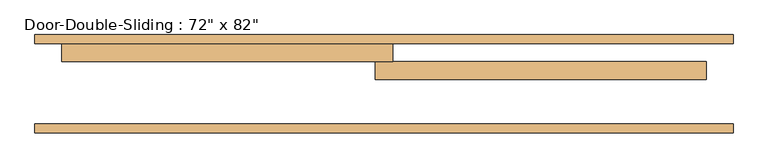
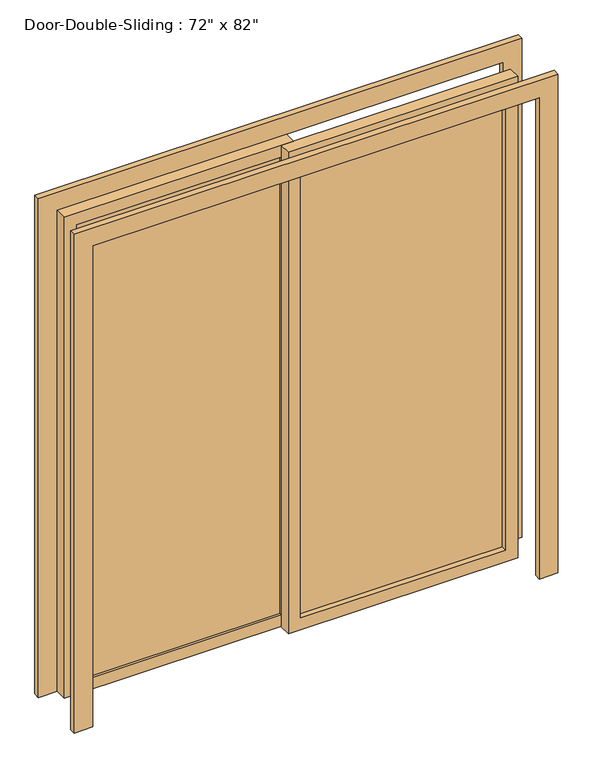
"""IFC4 building model written with IfcOpenShell, lengths in millimetres: door geometry."""

from ifc_helpers import new_model, si_unit, frame, origin, place, context, project, spatial, polyline, outline, extrude, source, transform, mapped, element, save


def door_b7c0cbe2(model_context):
    return source(origin(), model_context, "Body", "SweptSolid", [
        extrude(outline(polyline([(0.0, 990.6), (2159.0, 990.6), (2159.0, -990.6), (0.0, -990.6), (0.0, -914.4), (2082.8, -914.4), (2082.8, 914.4), (0.0, 914.4), (0.0, 990.6)])), frame((0.0, 241.3, 0.0), z_axis=(0.0, 1.0, 0.0), x_axis=(0.0, 0.0, 1.0)), (0.0, 0.0, 1.0), 25.4),
        extrude(outline(polyline([(0.0, -990.6), (0.0, -914.4), (2082.8, -914.4), (2082.8, 914.4), (0.0, 914.4), (0.0, 990.6), (2159.0, 990.6), (2159.0, -990.6), (0.0, -990.6)])), frame((0.0, -12.7, 0.0), z_axis=(0.0, 1.0, 0.0), x_axis=(0.0, 0.0, 1.0)), (0.0, 0.0, 1.0), 25.4),
        extrude(outline(polyline([(2082.8, 25.4), (2082.8, -914.4), (0.0, -914.4), (0.0, 25.4), (2082.8, 25.4)]), holes=[polyline([(2032.0, -25.4), (50.8, -25.4), (50.8, -863.6), (2032.0, -863.6), (2032.0, -25.4)])]), frame((0.0, 190.5, 0.0), z_axis=(0.0, 1.0, 0.0), x_axis=(0.0, 0.0, 1.0)), (0.0, 0.0, 1.0), 50.8),
        extrude(outline(polyline([(2082.8, -25.4), (0.0, -25.4), (0.0, 914.4), (2082.8, 914.4), (2082.8, -25.4)]), holes=[polyline([(2032.0, 25.4), (2032.0, 863.6), (50.8, 863.6), (50.8, 25.4), (2032.0, 25.4)])]), frame((0.0, 139.7, 0.0), z_axis=(0.0, 1.0, 0.0), x_axis=(0.0, 0.0, 1.0)), (0.0, 0.0, 1.0), 50.8),
        extrude(outline(polyline([(-25.4, 200.025), (-863.6, 200.025), (-863.6, 206.375), (-25.4, 206.375), (-25.4, 200.025)])), frame((0.0, 0.0, 50.8), z_axis=(0.0, 0.0, 1.0), x_axis=(1.0, 0.0, 0.0)), (0.0, 0.0, 1.0), 1981.2),
        extrude(outline(polyline([(25.4, 168.275), (863.6, 168.275), (863.6, 161.925), (25.4, 161.925), (25.4, 168.275)])), frame((0.0, 0.0, 50.8), z_axis=(0.0, 0.0, 1.0), x_axis=(1.0, 0.0, 0.0)), (0.0, 0.0, 1.0), 1981.2),
    ])


if __name__ == "__main__":
    model = new_model("IFC4")
    model_context = context("Model", 3, world=origin())
    ifc_project = project(units=[si_unit("LENGTHUNIT", "METRE", prefix="MILLI")], contexts=[model_context])
    site = spatial("IfcSite", under=ifc_project)
    building = spatial("IfcBuilding", under=site)
    placement = place(None, origin())
    door_shape = door_b7c0cbe2(model_context)
    element("IfcDoor", 1, ObjectType="Door-Double-Sliding : 72\" x 82\"", at=placement, inside=building, context=model_context, shape_type="MappedRepresentation", body=[
        mapped(door_shape, transform((0.0, 0.0, 0.0), x_axis=(1.0, 0.0, 0.0), y_axis=(0.0, 1.0, 0.0), z_axis=(0.0, 0.0, 1.0))),
    ])
    save(model, "model.ifc")

# Revit data of these elements
# Type "Door-Double-Sliding : 72\" x 82\""
#   Type Mark = "17"
#   Construction Type Id = "opn-d45"
#   Assembly Code = "C1020"
#   Analytic Construction = "Wood frame, double glass door "
#   Thickness = 0' - 2"
#   Thermal Resistance (R) = 1.8150 (h·ft²·°F)/BTU
#   Heat Transfer Coefficient (U) = 0.5510 BTU/(h·ft²·°F)
#   Height = 6' - 10"
#   Rail Width = 0' - 2"
#   Stiles = 0' - 2"
#   Trim Projection Ext = 0' - 1"
#   Trim Projection Int = 0' - 1"
#   Trim Width = 0' - 3"
#   Width = 6' - 0"
#   Define Thermal Properties by = 1
#   Glazing = Glass
#   Panel Material = Wood - Birch - Solid Stained Light Low Gloss
#   Trim Material = Paint - Sienna
#   Visual Light Transmittance = 0
#   Solar Heat Gain Coefficient = 0
#   Function = (empty or 0)
#   Wall Closure = (empty or 0)
# Element 1 (IfcDoor, "Door-Double-Sliding : 72\" x 82\"")
#   Materials on its faces: "Paint - Sienna", "Wood - Birch - Solid Stained Light Low Gloss", "Glass"
# Materials
#   "Glass": class "Glass", colour RGB 0 128 192, transparency 0.75, Description = "Soda Lime Glass", Cost = 0
#   "Wood - Birch - Solid Stained Light Low Gloss": class "Wood", colour RGB 210 159 95, transparency 0, Cost = 0
#   "Paint - Sienna": colour RGB 118 70 51, transparency 0, Cost = 0
